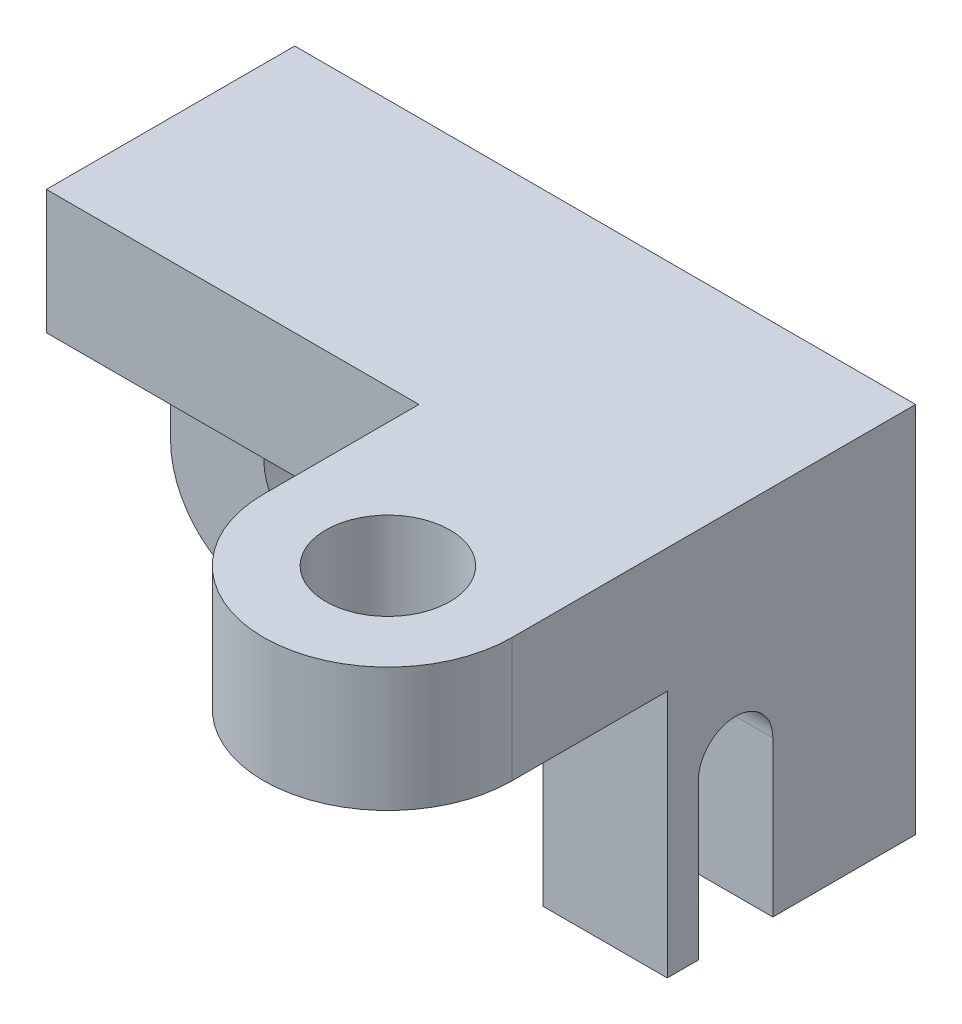
ISO-10303-21;
HEADER;
FILE_DESCRIPTION(('STEP AP214'),'2;1');
FILE_NAME('part.step','',(''),(''),'','','');
FILE_SCHEMA(('AUTOMOTIVE_DESIGN { 1 0 10303 214 1 1 1 1 }'));
ENDSEC;
DATA;
#1=APPLICATION_CONTEXT('core data for automotive mechanical design processes');
#2=APPLICATION_PROTOCOL_DEFINITION('international standard','automotive_design',2000,#1);
#3=PRODUCT_CONTEXT('',#1,'mechanical');
#4=PRODUCT('Part','Part','',(#3));
#5=PRODUCT_RELATED_PRODUCT_CATEGORY('part','',(#4));
#6=PRODUCT_DEFINITION_FORMATION('','',#4);
#7=PRODUCT_DEFINITION_CONTEXT('part definition',#1,'design');
#8=PRODUCT_DEFINITION('design','',#6,#7);
#9=PRODUCT_DEFINITION_SHAPE('','',#8);
#10=(LENGTH_UNIT() NAMED_UNIT(*) SI_UNIT(.MILLI.,.METRE.));
#11=(NAMED_UNIT(*) PLANE_ANGLE_UNIT() SI_UNIT($,.RADIAN.));
#12=(NAMED_UNIT(*) SI_UNIT($,.STERADIAN.) SOLID_ANGLE_UNIT());
#13=UNCERTAINTY_MEASURE_WITH_UNIT(LENGTH_MEASURE(1.E-05),#10,'distance_accuracy_value','');
#14=(GEOMETRIC_REPRESENTATION_CONTEXT(3) GLOBAL_UNCERTAINTY_ASSIGNED_CONTEXT((#13)) GLOBAL_UNIT_ASSIGNED_CONTEXT((#10,
#11,#12)) REPRESENTATION_CONTEXT('',''));
#15=CARTESIAN_POINT('',(0.,0.,0.));
#16=DIRECTION('',(0.,0.,1.));
#17=DIRECTION('',(1.,0.,0.));
#18=AXIS2_PLACEMENT_3D('',#15,#16,#17);
#19=CARTESIAN_POINT('',(-85.,15.,20.));
#20=DIRECTION('',(0.,0.,1.));
#21=DIRECTION('',(1.,0.,0.));
#22=AXIS2_PLACEMENT_3D('',#19,#20,#21);
#23=PLANE('',#22);
#24=CARTESIAN_POINT('',(-75.,20.,20.));
#25=DIRECTION('',(0.,0.,1.));
#26=DIRECTION('',(1.,0.,0.));
#27=AXIS2_PLACEMENT_3D('',#24,#25,#26);
#28=CIRCLE('',#27,9.99999999999999);
#29=CARTESIAN_POINT('',(-65.,20.,20.));
#30=VERTEX_POINT('',#29);
#31=EDGE_CURVE('E299',#30,#30,#28,.T.);
#32=ORIENTED_EDGE('',*,*,#31,.F.);
#33=EDGE_LOOP('',(#32));
#34=FACE_BOUND('',#33,.T.);
#35=DIRECTION('',(0.,1.,0.));
#36=VECTOR('',#35,1.);
#37=CARTESIAN_POINT('',(-20.,0.,20.));
#38=LINE('',#37,#36);
#39=CARTESIAN_POINT('',(-20.,0.,20.));
#40=VERTEX_POINT('',#39);
#41=CARTESIAN_POINT('',(-20.,40.,20.));
#42=VERTEX_POINT('',#41);
#43=EDGE_CURVE('E214',#40,#42,#38,.T.);
#44=ORIENTED_EDGE('',*,*,#43,.T.);
#45=DIRECTION('',(-1.,0.,0.));
#46=VECTOR('',#45,1.);
#47=CARTESIAN_POINT('',(-40.,40.,20.));
#48=LINE('',#47,#46);
#49=CARTESIAN_POINT('',(-100.,40.,20.));
#50=VERTEX_POINT('',#49);
#51=EDGE_CURVE('E269',#42,#50,#48,.T.);
#52=ORIENTED_EDGE('',*,*,#51,.T.);
#53=DIRECTION('',(0.,-1.,0.));
#54=VECTOR('',#53,1.);
#55=CARTESIAN_POINT('',(-100.,15.,20.));
#56=LINE('',#55,#54);
#57=CARTESIAN_POINT('',(-100.,15.,20.));
#58=VERTEX_POINT('',#57);
#59=EDGE_CURVE('E96',#50,#58,#56,.T.);
#60=ORIENTED_EDGE('',*,*,#59,.T.);
#61=CARTESIAN_POINT('',(-85.,15.,20.));
#62=DIRECTION('',(0.,0.,1.));
#63=DIRECTION('',(1.,0.,0.));
#64=AXIS2_PLACEMENT_3D('',#61,#62,#63);
#65=CIRCLE('',#64,15.);
#66=CARTESIAN_POINT('',(-85.,0.,20.));
#67=VERTEX_POINT('',#66);
#68=EDGE_CURVE('E65',#58,#67,#65,.T.);
#69=ORIENTED_EDGE('',*,*,#68,.T.);
#70=DIRECTION('',(1.,0.,0.));
#71=VECTOR('',#70,1.);
#72=CARTESIAN_POINT('',(0.,0.,20.));
#73=LINE('',#72,#71);
#74=EDGE_CURVE('E108',#67,#40,#73,.T.);
#75=ORIENTED_EDGE('',*,*,#74,.T.);
#76=EDGE_LOOP('',(#44,#52,#60,#69,#75));
#77=FACE_BOUND('',#76,.T.);
#78=ADVANCED_FACE('F44',(#34,#77),#23,.T.);
#79=CARTESIAN_POINT('',(0.,60.,20.));
#80=DIRECTION('',(-1.,0.,0.));
#81=DIRECTION('',(0.,0.,1.));
#82=AXIS2_PLACEMENT_3D('',#79,#80,#81);
#83=PLANE('',#82);
#84=DIRECTION('',(0.,0.,-1.));
#85=VECTOR('',#84,1.);
#86=CARTESIAN_POINT('',(0.,60.,20.));
#87=LINE('',#86,#85);
#88=CARTESIAN_POINT('',(0.,60.,65.));
#89=VERTEX_POINT('',#88);
#90=CARTESIAN_POINT('',(0.,60.,0.));
#91=VERTEX_POINT('',#90);
#92=EDGE_CURVE('E11',#89,#91,#87,.T.);
#93=ORIENTED_EDGE('',*,*,#92,.F.);
#94=DIRECTION('',(0.,1.,0.));
#95=VECTOR('',#94,1.);
#96=CARTESIAN_POINT('',(0.,40.,65.));
#97=LINE('',#96,#95);
#98=CARTESIAN_POINT('',(0.,40.,65.));
#99=VERTEX_POINT('',#98);
#100=EDGE_CURVE('E270',#99,#89,#97,.T.);
#101=ORIENTED_EDGE('',*,*,#100,.F.);
#102=DIRECTION('',(0.,0.,-1.));
#103=VECTOR('',#102,1.);
#104=CARTESIAN_POINT('',(0.,40.,20.));
#105=LINE('',#104,#103);
#106=CARTESIAN_POINT('',(0.,40.,40.));
#107=VERTEX_POINT('',#106);
#108=EDGE_CURVE('E280',#99,#107,#105,.T.);
#109=ORIENTED_EDGE('',*,*,#108,.T.);
#110=DIRECTION('',(0.,-1.,0.));
#111=VECTOR('',#110,1.);
#112=CARTESIAN_POINT('',(0.,40.,40.));
#113=LINE('',#112,#111);
#114=CARTESIAN_POINT('',(0.,0.,40.));
#115=VERTEX_POINT('',#114);
#116=EDGE_CURVE('E240',#107,#115,#113,.T.);
#117=ORIENTED_EDGE('',*,*,#116,.T.);
#118=DIRECTION('',(0.,0.,-1.));
#119=VECTOR('',#118,1.);
#120=CARTESIAN_POINT('',(0.,0.,40.));
#121=LINE('',#120,#119);
#122=CARTESIAN_POINT('',(0.,0.,35.));
#123=VERTEX_POINT('',#122);
#124=EDGE_CURVE('E239',#115,#123,#121,.T.);
#125=ORIENTED_EDGE('',*,*,#124,.T.);
#126=DIRECTION('',(0.,1.,0.));
#127=VECTOR('',#126,1.);
#128=CARTESIAN_POINT('',(0.,25.,35.));
#129=LINE('',#128,#127);
#130=CARTESIAN_POINT('',(0.,25.,35.));
#131=VERTEX_POINT('',#130);
#132=EDGE_CURVE('E210',#123,#131,#129,.T.);
#133=ORIENTED_EDGE('',*,*,#132,.T.);
#134=CARTESIAN_POINT('',(0.,25.,29.));
#135=DIRECTION('',(-1.,0.,0.));
#136=DIRECTION('',(0.,0.,-1.));
#137=AXIS2_PLACEMENT_3D('',#134,#135,#136);
#138=CIRCLE('',#137,6.);
#139=CARTESIAN_POINT('',(0.,25.,23.));
#140=VERTEX_POINT('',#139);
#141=EDGE_CURVE('E196',#131,#140,#138,.T.);
#142=ORIENTED_EDGE('',*,*,#141,.T.);
#143=DIRECTION('',(0.,-1.,0.));
#144=VECTOR('',#143,1.);
#145=CARTESIAN_POINT('',(0.,0.,23.));
#146=LINE('',#145,#144);
#147=CARTESIAN_POINT('',(0.,0.,23.));
#148=VERTEX_POINT('',#147);
#149=EDGE_CURVE('E110',#140,#148,#146,.T.);
#150=ORIENTED_EDGE('',*,*,#149,.T.);
#151=DIRECTION('',(0.,0.,-1.));
#152=VECTOR('',#151,1.);
#153=CARTESIAN_POINT('',(0.,0.,20.));
#154=LINE('',#153,#152);
#155=CARTESIAN_POINT('',(0.,0.,0.));
#156=VERTEX_POINT('',#155);
#157=EDGE_CURVE('E94',#148,#156,#154,.T.);
#158=ORIENTED_EDGE('',*,*,#157,.T.);
#159=DIRECTION('',(0.,1.,0.));
#160=VECTOR('',#159,1.);
#161=CARTESIAN_POINT('',(0.,60.,0.));
#162=LINE('',#161,#160);
#163=EDGE_CURVE('E104',#156,#91,#162,.T.);
#164=ORIENTED_EDGE('',*,*,#163,.T.);
#165=EDGE_LOOP('',(#93,#101,#109,#117,#125,#133,#142,#150,#158,#164));
#166=FACE_BOUND('',#165,.T.);
#167=ADVANCED_FACE('F50',(#166),#83,.F.);
#168=CARTESIAN_POINT('',(-100.,60.,20.));
#169=DIRECTION('',(0.,-1.,0.));
#170=DIRECTION('',(0.,0.,-1.));
#171=AXIS2_PLACEMENT_3D('',#168,#169,#170);
#172=PLANE('',#171);
#173=CARTESIAN_POINT('',(-20.,60.,65.));
#174=DIRECTION('',(0.,-1.,0.));
#175=DIRECTION('',(0.,0.,-1.));
#176=AXIS2_PLACEMENT_3D('',#173,#174,#175);
#177=CIRCLE('',#176,10.);
#178=CARTESIAN_POINT('',(-20.,60.,55.));
#179=VERTEX_POINT('',#178);
#180=EDGE_CURVE('E287',#179,#179,#177,.T.);
#181=ORIENTED_EDGE('',*,*,#180,.T.);
#182=EDGE_LOOP('',(#181));
#183=FACE_BOUND('',#182,.T.);
#184=DIRECTION('',(-1.,0.,0.));
#185=VECTOR('',#184,1.);
#186=CARTESIAN_POINT('',(-100.,60.,0.));
#187=LINE('',#186,#185);
#188=CARTESIAN_POINT('',(-100.,60.,0.));
#189=VERTEX_POINT('',#188);
#190=EDGE_CURVE('E115',#91,#189,#187,.T.);
#191=ORIENTED_EDGE('',*,*,#190,.T.);
#192=DIRECTION('',(0.,0.,-1.));
#193=VECTOR('',#192,1.);
#194=CARTESIAN_POINT('',(-100.,60.,20.));
#195=LINE('',#194,#193);
#196=CARTESIAN_POINT('',(-100.,60.,40.));
#197=VERTEX_POINT('',#196);
#198=EDGE_CURVE('E53',#197,#189,#195,.T.);
#199=ORIENTED_EDGE('',*,*,#198,.F.);
#200=DIRECTION('',(1.,0.,0.));
#201=VECTOR('',#200,1.);
#202=CARTESIAN_POINT('',(-100.,60.,40.));
#203=LINE('',#202,#201);
#204=CARTESIAN_POINT('',(-40.,60.,40.));
#205=VERTEX_POINT('',#204);
#206=EDGE_CURVE('E145',#197,#205,#203,.T.);
#207=ORIENTED_EDGE('',*,*,#206,.T.);
#208=DIRECTION('',(0.,0.,1.));
#209=VECTOR('',#208,1.);
#210=CARTESIAN_POINT('',(-40.,60.,65.));
#211=LINE('',#210,#209);
#212=CARTESIAN_POINT('',(-40.,60.,65.));
#213=VERTEX_POINT('',#212);
#214=EDGE_CURVE('E282',#205,#213,#211,.T.);
#215=ORIENTED_EDGE('',*,*,#214,.T.);
#216=CARTESIAN_POINT('',(-20.,60.,65.));
#217=DIRECTION('',(0.,1.,0.));
#218=DIRECTION('',(0.,0.,1.));
#219=AXIS2_PLACEMENT_3D('',#216,#217,#218);
#220=CIRCLE('',#219,20.);
#221=EDGE_CURVE('E278',#213,#89,#220,.T.);
#222=ORIENTED_EDGE('',*,*,#221,.T.);
#223=ORIENTED_EDGE('',*,*,#92,.T.);
#224=EDGE_LOOP('',(#191,#199,#207,#215,#222,#223));
#225=FACE_BOUND('',#224,.T.);
#226=ADVANCED_FACE('F136',(#183,#225),#172,.F.);
#227=CARTESIAN_POINT('',(-100.,15.,20.));
#228=DIRECTION('',(1.,0.,0.));
#229=DIRECTION('',(0.,0.,-1.));
#230=AXIS2_PLACEMENT_3D('',#227,#228,#229);
#231=PLANE('',#230);
#232=DIRECTION('',(0.,-1.,0.));
#233=VECTOR('',#232,1.);
#234=CARTESIAN_POINT('',(-100.,15.,0.));
#235=LINE('',#234,#233);
#236=CARTESIAN_POINT('',(-100.,15.,0.));
#237=VERTEX_POINT('',#236);
#238=EDGE_CURVE('E114',#189,#237,#235,.T.);
#239=ORIENTED_EDGE('',*,*,#238,.T.);
#240=DIRECTION('',(0.,0.,-1.));
#241=VECTOR('',#240,1.);
#242=CARTESIAN_POINT('',(-100.,15.,20.));
#243=LINE('',#242,#241);
#244=EDGE_CURVE('E123',#58,#237,#243,.T.);
#245=ORIENTED_EDGE('',*,*,#244,.F.);
#246=ORIENTED_EDGE('',*,*,#59,.F.);
#247=DIRECTION('',(0.,0.,1.));
#248=VECTOR('',#247,1.);
#249=CARTESIAN_POINT('',(-100.,40.,20.));
#250=LINE('',#249,#248);
#251=CARTESIAN_POINT('',(-100.,40.,40.));
#252=VERTEX_POINT('',#251);
#253=EDGE_CURVE('E272',#50,#252,#250,.T.);
#254=ORIENTED_EDGE('',*,*,#253,.T.);
#255=DIRECTION('',(0.,1.,0.));
#256=VECTOR('',#255,1.);
#257=CARTESIAN_POINT('',(-100.,40.,40.));
#258=LINE('',#257,#256);
#259=EDGE_CURVE('E134',#252,#197,#258,.T.);
#260=ORIENTED_EDGE('',*,*,#259,.T.);
#261=ORIENTED_EDGE('',*,*,#198,.T.);
#262=EDGE_LOOP('',(#239,#245,#246,#254,#260,#261));
#263=FACE_BOUND('',#262,.T.);
#264=ADVANCED_FACE('F128',(#263),#231,.F.);
#265=CARTESIAN_POINT('',(-85.,15.,20.));
#266=DIRECTION('',(0.,0.,-1.));
#267=DIRECTION('',(-1.,0.,0.));
#268=AXIS2_PLACEMENT_3D('',#265,#266,#267);
#269=CYLINDRICAL_SURFACE('',#268,15.);
#270=CARTESIAN_POINT('',(-85.,15.,0.));
#271=DIRECTION('',(0.,0.,1.));
#272=DIRECTION('',(1.,0.,0.));
#273=AXIS2_PLACEMENT_3D('',#270,#271,#272);
#274=CIRCLE('',#273,15.);
#275=CARTESIAN_POINT('',(-85.,0.,0.));
#276=VERTEX_POINT('',#275);
#277=EDGE_CURVE('E82',#237,#276,#274,.T.);
#278=ORIENTED_EDGE('',*,*,#277,.T.);
#279=DIRECTION('',(0.,0.,-1.));
#280=VECTOR('',#279,1.);
#281=CARTESIAN_POINT('',(-85.,0.,20.));
#282=LINE('',#281,#280);
#283=EDGE_CURVE('E93',#67,#276,#282,.T.);
#284=ORIENTED_EDGE('',*,*,#283,.F.);
#285=ORIENTED_EDGE('',*,*,#68,.F.);
#286=ORIENTED_EDGE('',*,*,#244,.T.);
#287=EDGE_LOOP('',(#278,#284,#285,#286));
#288=FACE_BOUND('',#287,.T.);
#289=ADVANCED_FACE('F330',(#288),#269,.T.);
#290=CARTESIAN_POINT('',(0.,0.,20.));
#291=DIRECTION('',(0.,1.,0.));
#292=DIRECTION('',(0.,0.,1.));
#293=AXIS2_PLACEMENT_3D('',#290,#291,#292);
#294=PLANE('',#293);
#295=DIRECTION('',(1.,0.,0.));
#296=VECTOR('',#295,1.);
#297=CARTESIAN_POINT('',(0.,0.,0.));
#298=LINE('',#297,#296);
#299=EDGE_CURVE('E90',#276,#156,#298,.T.);
#300=ORIENTED_EDGE('',*,*,#299,.T.);
#301=ORIENTED_EDGE('',*,*,#157,.F.);
#302=DIRECTION('',(1.,0.,0.));
#303=VECTOR('',#302,1.);
#304=CARTESIAN_POINT('',(-20.,0.,23.));
#305=LINE('',#304,#303);
#306=CARTESIAN_POINT('',(-20.,0.,23.));
#307=VERTEX_POINT('',#306);
#308=EDGE_CURVE('E113',#307,#148,#305,.T.);
#309=ORIENTED_EDGE('',*,*,#308,.F.);
#310=DIRECTION('',(0.,0.,-1.));
#311=VECTOR('',#310,1.);
#312=CARTESIAN_POINT('',(-20.,0.,20.));
#313=LINE('',#312,#311);
#314=EDGE_CURVE('E208',#307,#40,#313,.T.);
#315=ORIENTED_EDGE('',*,*,#314,.T.);
#316=ORIENTED_EDGE('',*,*,#74,.F.);
#317=ORIENTED_EDGE('',*,*,#283,.T.);
#318=EDGE_LOOP('',(#300,#301,#309,#315,#316,#317));
#319=FACE_BOUND('',#318,.T.);
#320=ADVANCED_FACE('F87',(#319),#294,.F.);
#321=CARTESIAN_POINT('',(-85.,15.,0.));
#322=DIRECTION('',(0.,0.,1.));
#323=DIRECTION('',(1.,0.,0.));
#324=AXIS2_PLACEMENT_3D('',#321,#322,#323);
#325=PLANE('',#324);
#326=CARTESIAN_POINT('',(-75.,20.,0.));
#327=DIRECTION('',(0.,0.,1.));
#328=DIRECTION('',(1.,0.,0.));
#329=AXIS2_PLACEMENT_3D('',#326,#327,#328);
#330=CIRCLE('',#329,9.99999999999999);
#331=CARTESIAN_POINT('',(-65.,20.,0.));
#332=VERTEX_POINT('',#331);
#333=EDGE_CURVE('E298',#332,#332,#330,.T.);
#334=ORIENTED_EDGE('',*,*,#333,.T.);
#335=EDGE_LOOP('',(#334));
#336=FACE_BOUND('',#335,.T.);
#337=ORIENTED_EDGE('',*,*,#163,.F.);
#338=ORIENTED_EDGE('',*,*,#299,.F.);
#339=ORIENTED_EDGE('',*,*,#277,.F.);
#340=ORIENTED_EDGE('',*,*,#238,.F.);
#341=ORIENTED_EDGE('',*,*,#190,.F.);
#342=EDGE_LOOP('',(#337,#338,#339,#340,#341));
#343=FACE_BOUND('',#342,.T.);
#344=ADVANCED_FACE('F109',(#336,#343),#325,.F.);
#345=CARTESIAN_POINT('',(-20.,0.,23.));
#346=DIRECTION('',(0.,0.,1.));
#347=DIRECTION('',(1.,0.,0.));
#348=AXIS2_PLACEMENT_3D('',#345,#346,#347);
#349=PLANE('',#348);
#350=ORIENTED_EDGE('',*,*,#149,.F.);
#351=DIRECTION('',(1.,0.,0.));
#352=VECTOR('',#351,1.);
#353=CARTESIAN_POINT('',(-20.,25.,23.));
#354=LINE('',#353,#352);
#355=CARTESIAN_POINT('',(-20.,25.,23.));
#356=VERTEX_POINT('',#355);
#357=EDGE_CURVE('E120',#356,#140,#354,.T.);
#358=ORIENTED_EDGE('',*,*,#357,.F.);
#359=DIRECTION('',(0.,-1.,0.));
#360=VECTOR('',#359,1.);
#361=CARTESIAN_POINT('',(-20.,0.,23.));
#362=LINE('',#361,#360);
#363=EDGE_CURVE('E223',#356,#307,#362,.T.);
#364=ORIENTED_EDGE('',*,*,#363,.T.);
#365=ORIENTED_EDGE('',*,*,#308,.T.);
#366=EDGE_LOOP('',(#350,#358,#364,#365));
#367=FACE_BOUND('',#366,.T.);
#368=ADVANCED_FACE('F209',(#367),#349,.T.);
#369=CARTESIAN_POINT('',(-20.,25.,29.));
#370=DIRECTION('',(1.,0.,0.));
#371=DIRECTION('',(0.,0.,-1.));
#372=AXIS2_PLACEMENT_3D('',#369,#370,#371);
#373=CYLINDRICAL_SURFACE('',#372,6.);
#374=ORIENTED_EDGE('',*,*,#141,.F.);
#375=DIRECTION('',(1.,0.,0.));
#376=VECTOR('',#375,1.);
#377=CARTESIAN_POINT('',(-20.,25.,35.));
#378=LINE('',#377,#376);
#379=CARTESIAN_POINT('',(-20.,25.,35.));
#380=VERTEX_POINT('',#379);
#381=EDGE_CURVE('E205',#380,#131,#378,.T.);
#382=ORIENTED_EDGE('',*,*,#381,.F.);
#383=CARTESIAN_POINT('',(-20.,25.,29.));
#384=DIRECTION('',(-1.,0.,0.));
#385=DIRECTION('',(0.,0.,-1.));
#386=AXIS2_PLACEMENT_3D('',#383,#384,#385);
#387=CIRCLE('',#386,6.);
#388=EDGE_CURVE('E197',#380,#356,#387,.T.);
#389=ORIENTED_EDGE('',*,*,#388,.T.);
#390=ORIENTED_EDGE('',*,*,#357,.T.);
#391=EDGE_LOOP('',(#374,#382,#389,#390));
#392=FACE_BOUND('',#391,.T.);
#393=ADVANCED_FACE('F193',(#392),#373,.F.);
#394=CARTESIAN_POINT('',(-20.,25.,35.));
#395=DIRECTION('',(0.,0.,-1.));
#396=DIRECTION('',(-1.,0.,0.));
#397=AXIS2_PLACEMENT_3D('',#394,#395,#396);
#398=PLANE('',#397);
#399=ORIENTED_EDGE('',*,*,#132,.F.);
#400=DIRECTION('',(1.,0.,0.));
#401=VECTOR('',#400,1.);
#402=CARTESIAN_POINT('',(-20.,0.,35.));
#403=LINE('',#402,#401);
#404=CARTESIAN_POINT('',(-20.,0.,35.));
#405=VERTEX_POINT('',#404);
#406=EDGE_CURVE('E218',#405,#123,#403,.T.);
#407=ORIENTED_EDGE('',*,*,#406,.F.);
#408=DIRECTION('',(0.,1.,0.));
#409=VECTOR('',#408,1.);
#410=CARTESIAN_POINT('',(-20.,25.,35.));
#411=LINE('',#410,#409);
#412=EDGE_CURVE('E231',#405,#380,#411,.T.);
#413=ORIENTED_EDGE('',*,*,#412,.T.);
#414=ORIENTED_EDGE('',*,*,#381,.T.);
#415=EDGE_LOOP('',(#399,#407,#413,#414));
#416=FACE_BOUND('',#415,.T.);
#417=ADVANCED_FACE('F255',(#416),#398,.T.);
#418=CARTESIAN_POINT('',(-20.,0.,40.));
#419=DIRECTION('',(0.,-1.,0.));
#420=DIRECTION('',(0.,0.,-1.));
#421=AXIS2_PLACEMENT_3D('',#418,#419,#420);
#422=PLANE('',#421);
#423=ORIENTED_EDGE('',*,*,#124,.F.);
#424=DIRECTION('',(1.,0.,0.));
#425=VECTOR('',#424,1.);
#426=CARTESIAN_POINT('',(-20.,0.,40.));
#427=LINE('',#426,#425);
#428=CARTESIAN_POINT('',(-20.,0.,40.));
#429=VERTEX_POINT('',#428);
#430=EDGE_CURVE('E219',#429,#115,#427,.T.);
#431=ORIENTED_EDGE('',*,*,#430,.F.);
#432=DIRECTION('',(0.,0.,-1.));
#433=VECTOR('',#432,1.);
#434=CARTESIAN_POINT('',(-20.,0.,40.));
#435=LINE('',#434,#433);
#436=EDGE_CURVE('E247',#429,#405,#435,.T.);
#437=ORIENTED_EDGE('',*,*,#436,.T.);
#438=ORIENTED_EDGE('',*,*,#406,.T.);
#439=EDGE_LOOP('',(#423,#431,#437,#438));
#440=FACE_BOUND('',#439,.T.);
#441=ADVANCED_FACE('F244',(#440),#422,.T.);
#442=CARTESIAN_POINT('',(-20.,40.,40.));
#443=DIRECTION('',(0.,0.,1.));
#444=DIRECTION('',(1.,0.,0.));
#445=AXIS2_PLACEMENT_3D('',#442,#443,#444);
#446=PLANE('',#445);
#447=ORIENTED_EDGE('',*,*,#116,.F.);
#448=DIRECTION('',(1.,0.,0.));
#449=VECTOR('',#448,1.);
#450=CARTESIAN_POINT('',(-20.,40.,40.));
#451=LINE('',#450,#449);
#452=CARTESIAN_POINT('',(-20.,40.,40.));
#453=VERTEX_POINT('',#452);
#454=EDGE_CURVE('E224',#453,#107,#451,.T.);
#455=ORIENTED_EDGE('',*,*,#454,.F.);
#456=DIRECTION('',(0.,-1.,0.));
#457=VECTOR('',#456,1.);
#458=CARTESIAN_POINT('',(-20.,40.,40.));
#459=LINE('',#458,#457);
#460=EDGE_CURVE('E253',#453,#429,#459,.T.);
#461=ORIENTED_EDGE('',*,*,#460,.T.);
#462=ORIENTED_EDGE('',*,*,#430,.T.);
#463=EDGE_LOOP('',(#447,#455,#461,#462));
#464=FACE_BOUND('',#463,.T.);
#465=ADVANCED_FACE('F322',(#464),#446,.T.);
#466=CARTESIAN_POINT('',(-20.,25.,29.));
#467=DIRECTION('',(1.,0.,0.));
#468=DIRECTION('',(0.,0.,-1.));
#469=AXIS2_PLACEMENT_3D('',#466,#467,#468);
#470=PLANE('',#469);
#471=ORIENTED_EDGE('',*,*,#314,.F.);
#472=ORIENTED_EDGE('',*,*,#363,.F.);
#473=ORIENTED_EDGE('',*,*,#388,.F.);
#474=ORIENTED_EDGE('',*,*,#412,.F.);
#475=ORIENTED_EDGE('',*,*,#436,.F.);
#476=ORIENTED_EDGE('',*,*,#460,.F.);
#477=DIRECTION('',(0.,0.,1.));
#478=VECTOR('',#477,1.);
#479=CARTESIAN_POINT('',(-20.,40.,20.));
#480=LINE('',#479,#478);
#481=EDGE_CURVE('E256',#42,#453,#480,.T.);
#482=ORIENTED_EDGE('',*,*,#481,.F.);
#483=ORIENTED_EDGE('',*,*,#43,.F.);
#484=EDGE_LOOP('',(#471,#472,#473,#474,#475,#476,#482,#483));
#485=FACE_BOUND('',#484,.T.);
#486=ADVANCED_FACE('F229',(#485),#470,.F.);
#487=CARTESIAN_POINT('',(-100.,40.,40.));
#488=DIRECTION('',(0.,0.,1.));
#489=DIRECTION('',(1.,0.,0.));
#490=AXIS2_PLACEMENT_3D('',#487,#488,#489);
#491=PLANE('',#490);
#492=ORIENTED_EDGE('',*,*,#206,.F.);
#493=ORIENTED_EDGE('',*,*,#259,.F.);
#494=DIRECTION('',(1.,0.,0.));
#495=VECTOR('',#494,1.);
#496=CARTESIAN_POINT('',(-100.,40.,40.));
#497=LINE('',#496,#495);
#498=CARTESIAN_POINT('',(-40.,40.,40.));
#499=VERTEX_POINT('',#498);
#500=EDGE_CURVE('E262',#252,#499,#497,.T.);
#501=ORIENTED_EDGE('',*,*,#500,.T.);
#502=DIRECTION('',(0.,1.,0.));
#503=VECTOR('',#502,1.);
#504=CARTESIAN_POINT('',(-40.,40.,40.));
#505=LINE('',#504,#503);
#506=EDGE_CURVE('E241',#499,#205,#505,.T.);
#507=ORIENTED_EDGE('',*,*,#506,.T.);
#508=EDGE_LOOP('',(#492,#493,#501,#507));
#509=FACE_BOUND('',#508,.T.);
#510=ADVANCED_FACE('F348',(#509),#491,.T.);
#511=CARTESIAN_POINT('',(0.,40.,0.));
#512=DIRECTION('',(0.,1.,0.));
#513=DIRECTION('',(0.,0.,1.));
#514=AXIS2_PLACEMENT_3D('',#511,#512,#513);
#515=PLANE('',#514);
#516=CARTESIAN_POINT('',(-20.,40.,65.));
#517=DIRECTION('',(0.,-1.,0.));
#518=DIRECTION('',(0.,0.,-1.));
#519=AXIS2_PLACEMENT_3D('',#516,#517,#518);
#520=CIRCLE('',#519,10.);
#521=CARTESIAN_POINT('',(-20.,40.,55.));
#522=VERTEX_POINT('',#521);
#523=EDGE_CURVE('E291',#522,#522,#520,.T.);
#524=ORIENTED_EDGE('',*,*,#523,.F.);
#525=EDGE_LOOP('',(#524));
#526=FACE_BOUND('',#525,.T.);
#527=ORIENTED_EDGE('',*,*,#51,.F.);
#528=ORIENTED_EDGE('',*,*,#481,.T.);
#529=ORIENTED_EDGE('',*,*,#454,.T.);
#530=ORIENTED_EDGE('',*,*,#108,.F.);
#531=CARTESIAN_POINT('',(-20.,40.,65.));
#532=DIRECTION('',(0.,1.,0.));
#533=DIRECTION('',(0.,0.,1.));
#534=AXIS2_PLACEMENT_3D('',#531,#532,#533);
#535=CIRCLE('',#534,20.);
#536=CARTESIAN_POINT('',(-40.,40.,65.));
#537=VERTEX_POINT('',#536);
#538=EDGE_CURVE('E290',#537,#99,#535,.T.);
#539=ORIENTED_EDGE('',*,*,#538,.F.);
#540=DIRECTION('',(0.,0.,1.));
#541=VECTOR('',#540,1.);
#542=CARTESIAN_POINT('',(-40.,40.,65.));
#543=LINE('',#542,#541);
#544=EDGE_CURVE('E283',#499,#537,#543,.T.);
#545=ORIENTED_EDGE('',*,*,#544,.F.);
#546=ORIENTED_EDGE('',*,*,#500,.F.);
#547=ORIENTED_EDGE('',*,*,#253,.F.);
#548=EDGE_LOOP('',(#527,#528,#529,#530,#539,#545,#546,#547));
#549=FACE_BOUND('',#548,.T.);
#550=ADVANCED_FACE('F341',(#526,#549),#515,.F.);
#551=CARTESIAN_POINT('',(-40.,40.,65.));
#552=DIRECTION('',(-1.,0.,0.));
#553=DIRECTION('',(0.,0.,1.));
#554=AXIS2_PLACEMENT_3D('',#551,#552,#553);
#555=PLANE('',#554);
#556=ORIENTED_EDGE('',*,*,#214,.F.);
#557=ORIENTED_EDGE('',*,*,#506,.F.);
#558=ORIENTED_EDGE('',*,*,#544,.T.);
#559=DIRECTION('',(0.,1.,0.));
#560=VECTOR('',#559,1.);
#561=CARTESIAN_POINT('',(-40.,40.,65.));
#562=LINE('',#561,#560);
#563=EDGE_CURVE('E274',#537,#213,#562,.T.);
#564=ORIENTED_EDGE('',*,*,#563,.T.);
#565=EDGE_LOOP('',(#556,#557,#558,#564));
#566=FACE_BOUND('',#565,.T.);
#567=ADVANCED_FACE('F350',(#566),#555,.T.);
#568=CARTESIAN_POINT('',(-20.,40.,65.));
#569=DIRECTION('',(0.,1.,0.));
#570=DIRECTION('',(0.,0.,1.));
#571=AXIS2_PLACEMENT_3D('',#568,#569,#570);
#572=CYLINDRICAL_SURFACE('',#571,20.);
#573=ORIENTED_EDGE('',*,*,#221,.F.);
#574=ORIENTED_EDGE('',*,*,#563,.F.);
#575=ORIENTED_EDGE('',*,*,#538,.T.);
#576=ORIENTED_EDGE('',*,*,#100,.T.);
#577=EDGE_LOOP('',(#573,#574,#575,#576));
#578=FACE_BOUND('',#577,.T.);
#579=ADVANCED_FACE('F338',(#578),#572,.T.);
#580=CARTESIAN_POINT('',(-20.,60.,65.));
#581=DIRECTION('',(0.,-1.,0.));
#582=DIRECTION('',(0.,0.,-1.));
#583=AXIS2_PLACEMENT_3D('',#580,#581,#582);
#584=CYLINDRICAL_SURFACE('',#583,10.);
#585=ORIENTED_EDGE('',*,*,#180,.F.);
#586=EDGE_LOOP('',(#585));
#587=FACE_BOUND('',#586,.T.);
#588=ORIENTED_EDGE('',*,*,#523,.T.);
#589=EDGE_LOOP('',(#588));
#590=FACE_BOUND('',#589,.T.);
#591=ADVANCED_FACE('F307',(#587,#590),#584,.F.);
#592=CARTESIAN_POINT('',(-75.,20.,0.));
#593=DIRECTION('',(0.,0.,1.));
#594=DIRECTION('',(1.,0.,0.));
#595=AXIS2_PLACEMENT_3D('',#592,#593,#594);
#596=CYLINDRICAL_SURFACE('',#595,9.99999999999999);
#597=ORIENTED_EDGE('',*,*,#333,.F.);
#598=EDGE_LOOP('',(#597));
#599=FACE_BOUND('',#598,.T.);
#600=ORIENTED_EDGE('',*,*,#31,.T.);
#601=EDGE_LOOP('',(#600));
#602=FACE_BOUND('',#601,.T.);
#603=ADVANCED_FACE('F306',(#599,#602),#596,.F.);
#604=CLOSED_SHELL('',(#78,#167,#226,#264,#289,#320,#344,#368,#393,#417,#441,#465,#486,#510,#550,
#567,#579,#591,#603));
#605=MANIFOLD_SOLID_BREP('B2',#604);
#606=ADVANCED_BREP_SHAPE_REPRESENTATION('',(#18,#605),#14);
#607=SHAPE_DEFINITION_REPRESENTATION(#9,#606);
ENDSEC;
END-ISO-10303-21;
